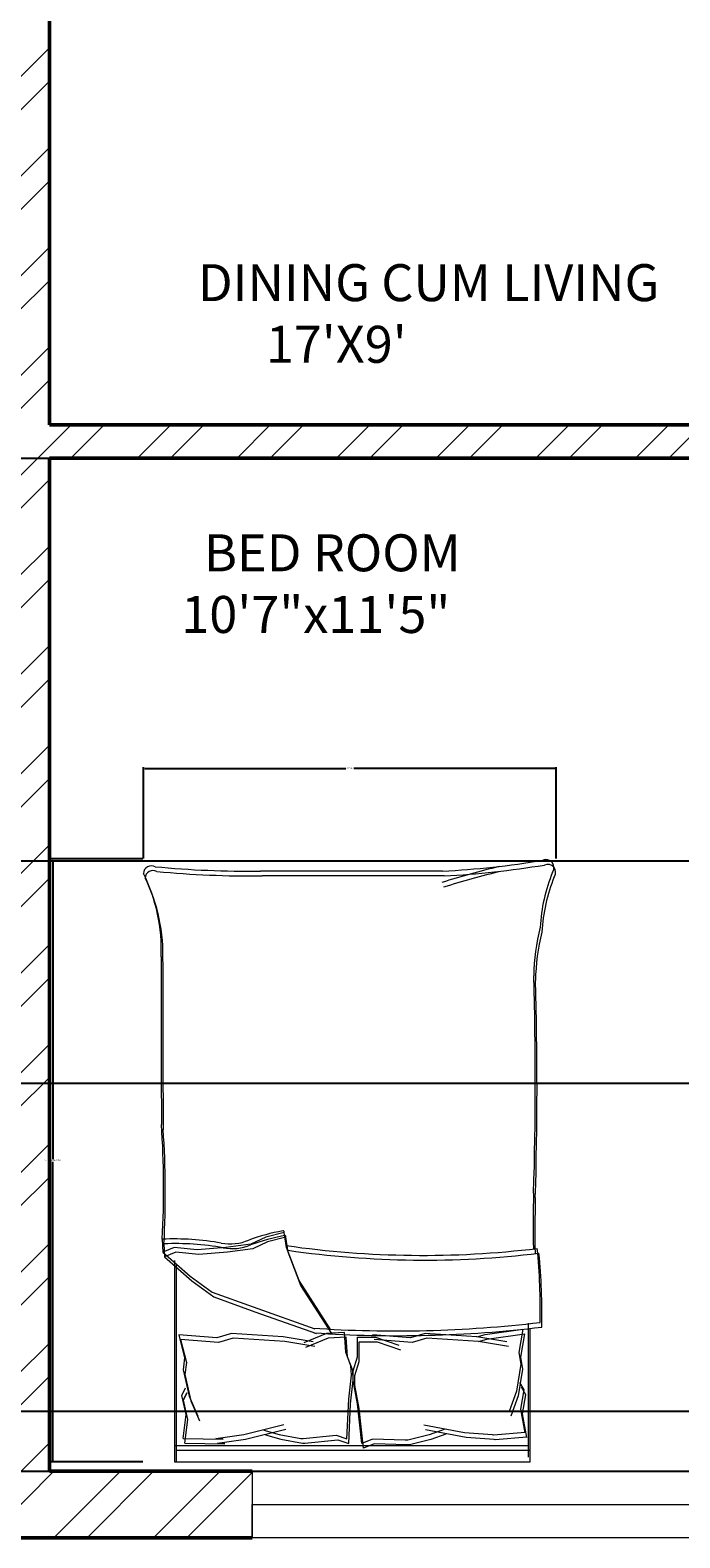
# Model space of a CAD drawing. Units: inches. Extents: x 2310 to 2937, y 1113 to 2410.
# Tile 10 of 23: x 2609 to 2697, y 1737 to 1940. Entities that reach past the tile are written whole.
import ezdxf

# ---------------------------------------------------------------- set-up
doc = ezdxf.new("R2010")
doc.units = ezdxf.units.IN
for name, color, linetype, lineweight in [('A-ANNO-DIMS', 2, 'Continuous', 18), ('A-AREA-IDEN', 7, 'Continuous', 18), ('A-FURN', 8, 'Continuous', 18), ('A-GLAZ', 191, 'Continuous', 20), ('A-WALL', 7, 'Continuous', 50), ('A-WALL-PATT', 85, 'Continuous', 13)]:
    doc.layers.add(name, color=color, linetype=linetype, lineweight=lineweight)
doc.styles.get("Standard").update_dxf_attribs({"font": 'arial.ttf'})
doc.dimstyles.get("Standard").update_dxf_attribs({"dimtxt": 0.18, "dimasz": 0.18, "dimexe": 0.18, "dimexo": 0.0625, "dimgap": 0.09, "dimtad": 0, "dimtih": 1, "dimtoh": 1, "dimdec": 4, "dimzin": 0, "dimdsep": 46, "dimtxsty": 'Standard', "dimcen": 0.09, "dimadec": 0, "dimazin": 0, "dimtfac": 1, "dimtdec": 4, "dimtofl": 0, "dimtmove": 0, "dimatfit": 3, "dimfxl": 1, "dimtolj": 1, "dimtzin": 0, "dimarcsym": 0})

# ---------------------------------------------------------------- blocks, each defined once
blk = doc.blocks.new('BED-DOUBLE')
for p, q in [((3.56, 63.44), (3.56, 81.55)), ((3.56, 63.44), (3.56, 81.55)), ((3.56, 81.55), (51.58, 81.55)), ((51.35, 81.55), (51.35, 54.94)), ((51.35, 81.55), (51.35, 54.94)), ((51.58, 81.55), (51.58, 80.91)), ((3.56, 80.01), (51.35, 80.01)), ((3.56, 80.01), (51.35, 80.01)), ((3.79, 62.8), (3.79, 80.91)), ((3.79, 62.8), (3.79, 80.91)), ((24.62, 79.1), (26.07, 79.68)), ((24.62, 79.1), (26.07, 79.68)), ((26.07, 79.68), (26.65, 74.33)), ((26.07, 79.68), (26.65, 74.33)), ((51.58, 80.91), (51.58, 54.3)), ((51.58, 80.91), (51.58, 54.3)), ((3.79, 79.38), (51.58, 79.38)), ((3.79, 79.38), (51.58, 79.38)), ((3.98, 78.21), (8.27, 78.54)), ((3.98, 78.23), (4.56, 75.05)), ((3.98, 78.23), (4.56, 75.05)), ((3.99, 78.21), (8.27, 78.54)), ((4.21, 77.57), (8.49, 77.9)), ((4.21, 77.57), (8.49, 77.9)), ((4.21, 77.59), (4.79, 74.41)), ((4.21, 77.59), (4.79, 74.41)), ((8.27, 78.54), (8.37, 78.52)), ((8.27, 78.54), (8.37, 78.52)), ((8.37, 78.52), (12.19, 78.23)), ((8.37, 78.52), (12.19, 78.23)), ((8.49, 77.9), (8.6, 77.88)), ((8.49, 77.9), (8.6, 77.88)), ((8.6, 77.88), (12.42, 77.59)), ((8.6, 77.88), (12.42, 77.59)), ((12.19, 78.23), (17.69, 77.22)), ((12.19, 78.23), (17.69, 77.22)), ((12.42, 77.59), (17.92, 76.58)), ((12.42, 77.59), (17.92, 76.58)), ((14.94, 77.8), (16.97, 78.52)), ((14.94, 77.8), (16.96, 78.52)), ((15.17, 77.16), (17.19, 77.88)), ((15.17, 77.16), (17.19, 77.88)), ((16.96, 78.52), (19.86, 79.24)), ((16.97, 78.52), (19.86, 79.24)), ((17.19, 77.88), (20.08, 78.61)), ((17.19, 77.88), (20.08, 78.61)), ((19.86, 79.24), (20.18, 79.24)), ((19.86, 79.24), (20.18, 79.24)), ((20.08, 78.61), (20.41, 78.61)), ((20.08, 78.61), (20.41, 78.61)), ((20.18, 79.24), (24.62, 79.1)), ((20.18, 79.24), (24.62, 79.1)), ((20.41, 78.61), (24.85, 78.46)), ((20.41, 78.61), (24.85, 78.46)), ((24.85, 78.46), (26.3, 79.04)), ((24.85, 78.46), (26.3, 79.04)), ((26.3, 79.04), (26.88, 73.69)), ((26.3, 79.04), (26.88, 73.69)), ((28.06, 79.06), (27.82, 73.68)), ((28.06, 79.06), (27.82, 73.68)), ((28.29, 78.42), (28.05, 73.04)), ((28.29, 78.42), (28.05, 73.04)), ((29.54, 78.57), (28.06, 79.06)), ((29.54, 78.57), (28.06, 79.06)), ((29.77, 77.93), (28.29, 78.42)), ((29.77, 77.93), (28.29, 78.42)), ((33.97, 78.99), (29.54, 78.57)), ((33.97, 78.99), (29.54, 78.57)), ((34.2, 78.35), (29.77, 77.93)), ((34.2, 78.35), (29.77, 77.93)), ((34.29, 79.01), (33.97, 78.99)), ((34.29, 79.01), (33.97, 78.99)), ((34.52, 78.37), (34.2, 78.35)), ((34.52, 78.37), (34.2, 78.35)), ((37.22, 78.47), (34.29, 79.01)), ((37.22, 78.47), (34.29, 79.01)), ((37.45, 77.83), (34.52, 78.37)), ((37.45, 77.83), (34.52, 78.37)), ((42, 78.48), (36.58, 77.13)), ((42, 78.48), (36.58, 77.13)), ((42.23, 77.84), (36.81, 76.49)), ((42.23, 77.84), (36.81, 76.49)), ((39.29, 77.87), (37.22, 78.47)), ((39.29, 77.87), (37.22, 78.47)), ((39.52, 77.24), (37.45, 77.83)), ((39.51, 77.24), (37.45, 77.83)), ((45.8, 79.01), (42, 78.48)), ((45.8, 79.01), (42, 78.48)), ((46.03, 78.37), (42.23, 77.84)), ((46.03, 78.37), (42.23, 77.84)), ((50.2, 78.99), (44.8, 79.09)), ((44.8, 79.09), (45.8, 79.01)), ((50.2, 78.99), (44.8, 79.09)), ((44.8, 79.09), (45.8, 79.01)), ((50.43, 78.35), (45.02, 78.45)), ((45.02, 78.45), (46.03, 78.37)), ((50.43, 78.35), (45.02, 78.45)), ((45.02, 78.45), (46.03, 78.37)), ((50.2, 78.99), (49.82, 75.78)), ((50.2, 78.99), (49.82, 75.78)), ((50.43, 78.35), (50.05, 75.14)), ((50.43, 78.35), (50.05, 75.14)), ((49.4, 73.29), (48.21, 75.97)), ((49.4, 73.29), (48.21, 75.97)), ((49.82, 75.78), (50.42, 73.21)), ((49.82, 75.78), (50.41, 73.21)), ((4.56, 75.05), (4.13, 72.45)), ((4.56, 75.05), (4.13, 72.45)), ((4.79, 74.41), (4.35, 71.81)), ((4.79, 74.41), (4.35, 71.81)), ((5.14, 72.59), (6.15, 75.34)), ((5.14, 72.59), (6.15, 75.34)), ((5.37, 71.95), (6.38, 74.7)), ((5.37, 71.95), (6.38, 74.7)), ((26.65, 74.33), (27.23, 71.15)), ((26.65, 74.33), (27.23, 71.15)), ((26.88, 73.69), (27.45, 70.51)), ((26.88, 73.69), (27.45, 70.51)), ((27.82, 73.68), (27.44, 70.47)), ((27.82, 73.68), (27.44, 70.47)), ((49.62, 72.65), (48.44, 75.33)), ((49.62, 72.65), (48.44, 75.33)), ((50.05, 75.14), (50.64, 72.57)), ((50.05, 75.14), (50.64, 72.57)), ((4.13, 72.45), (4.7, 71.44)), ((4.13, 72.45), (4.7, 71.44)), ((4.35, 71.81), (4.93, 70.8)), ((4.35, 71.81), (4.93, 70.8)), ((4.56, 68.98), (5.14, 72.59)), ((4.56, 68.98), (5.14, 72.59)), ((4.79, 68.34), (5.37, 71.95)), ((4.79, 68.34), (5.37, 71.95)), ((28.05, 73.04), (27.67, 69.83)), ((28.05, 73.04), (27.67, 69.83)), ((50.2, 69.72), (49.4, 73.29)), ((50.2, 69.72), (49.4, 73.29)), ((50.43, 69.08), (49.62, 72.65)), ((50.43, 69.08), (49.62, 72.65)), ((50.42, 73.21), (49.9, 72.16)), ((50.41, 73.21), (49.9, 72.16)), ((50.64, 72.57), (50.13, 71.52)), ((50.64, 72.57), (50.13, 71.52)), ((27.23, 69.85), (26.65, 67.97)), ((27.23, 69.85), (26.65, 67.97)), ((27.23, 71.15), (27.23, 69.85)), ((27.23, 71.15), (27.23, 69.85)), ((27.44, 70.47), (27.52, 69.17)), ((27.44, 70.47), (27.52, 69.17)), ((27.45, 70.51), (27.45, 69.21)), ((27.45, 70.51), (27.45, 69.21)), ((27.67, 69.83), (27.75, 68.53)), ((27.67, 69.83), (27.75, 68.53)), ((50.01, 68.11), (50.2, 69.72)), ((50.01, 68.11), (50.2, 69.72)), ((4.27, 64.21), (4.85, 67.39)), ((4.27, 64.21), (4.85, 67.39)), ((4.85, 67.39), (4.56, 68.98)), ((4.85, 67.39), (4.56, 68.98)), ((5.08, 66.75), (4.79, 68.34)), ((5.08, 66.75), (4.79, 68.34)), ((26.65, 67.97), (26.65, 65.29)), ((26.65, 67.97), (26.65, 65.29)), ((27.45, 69.21), (26.88, 67.33)), ((27.45, 69.21), (26.88, 67.33)), ((26.88, 67.33), (26.88, 64.65)), ((26.88, 67.33), (26.88, 64.65)), ((27.52, 69.17), (28.22, 67.33)), ((27.52, 69.17), (28.22, 67.33)), ((27.75, 68.53), (28.45, 66.69)), ((27.75, 68.53), (28.44, 66.69)), ((28.22, 67.33), (28.38, 64.66)), ((28.22, 67.33), (28.38, 64.66)), ((50.78, 64.98), (50.01, 68.11)), ((50.78, 64.98), (50.01, 68.11)), ((50.24, 67.48), (50.43, 69.08)), ((50.24, 67.48), (50.43, 69.08)), ((51.01, 64.34), (50.24, 67.48)), ((51.01, 64.34), (50.24, 67.48)), ((4.5, 63.57), (5.08, 66.75)), ((4.5, 63.57), (5.08, 66.75)), ((6.47, 65.92), (10.5, 65.25)), ((6.47, 65.92), (10.5, 65.25)), ((6.7, 65.28), (10.73, 64.61)), ((6.7, 65.28), (10.73, 64.61)), ((10.5, 65.25), (9.37, 64.93)), ((10.5, 65.25), (9.37, 64.93)), ((10.5, 65.25), (17.51, 64.82)), ((10.5, 65.25), (17.51, 64.82)), ((17.51, 64.82), (19.47, 65.38)), ((17.51, 64.82), (19.47, 65.38)), ((19.47, 65.38), (24.6, 64.98)), ((19.47, 65.38), (24.6, 64.98)), ((24.19, 65.29), (21.04, 66.38)), ((24.19, 65.29), (21.05, 66.38)), ((24.42, 64.65), (21.27, 65.74)), ((24.42, 64.65), (21.27, 65.74)), ((26.65, 65.29), (24.19, 65.29)), ((26.65, 65.29), (24.19, 65.29)), ((28.44, 66.69), (28.61, 64.02)), ((28.45, 66.69), (28.61, 64.02)), ((30.84, 64.81), (33.91, 66.09)), ((30.84, 64.81), (33.91, 66.09)), ((31.06, 64.17), (34.14, 65.45)), ((31.07, 64.17), (34.14, 65.45)), ((32.65, 65.92), (36.68, 65.25)), ((32.65, 65.92), (36.68, 65.25)), ((32.88, 65.28), (36.91, 64.61)), ((32.88, 65.28), (36.91, 64.61)), ((36.68, 65.25), (43.69, 64.82)), ((36.68, 65.25), (43.69, 64.82)), ((43.69, 64.82), (45.65, 65.38)), ((43.69, 64.82), (45.65, 65.38)), ((45.65, 65.38), (50.78, 64.98)), ((45.65, 65.38), (50.78, 64.98)), ((9.37, 64.93), (4.27, 64.21)), ((9.37, 64.93), (4.27, 64.21)), ((9.6, 64.29), (4.5, 63.57)), ((9.6, 64.29), (4.5, 63.57)), ((10.73, 64.61), (9.6, 64.29)), ((10.73, 64.61), (9.6, 64.29)), ((10.73, 64.61), (17.74, 64.18)), ((10.73, 64.61), (17.74, 64.18)), ((17.74, 64.18), (19.7, 64.74)), ((17.74, 64.18), (19.7, 64.74)), ((19.7, 64.74), (24.83, 64.34)), ((19.7, 64.74), (24.83, 64.34)), ((26.88, 64.65), (24.42, 64.65)), ((26.88, 64.65), (24.42, 64.65)), ((28.38, 64.66), (30.84, 64.81)), ((28.38, 64.66), (30.84, 64.81)), ((28.61, 64.02), (31.07, 64.17)), ((28.61, 64.02), (31.06, 64.17)), ((30.35, 64.17), (34.54, 57.67)), ((30.35, 64.17), (34.54, 57.67)), ((30.57, 63.53), (34.76, 57.03)), ((30.57, 63.53), (34.76, 57.03)), ((40.73, 61.23), (32.39, 64.17)), ((40.73, 61.23), (32.39, 64.17)), ((40.96, 60.59), (32.62, 63.53)), ((40.96, 60.59), (32.62, 63.53)), ((36.91, 64.61), (43.92, 64.18)), ((36.91, 64.61), (43.92, 64.18)), ((43.92, 64.18), (45.88, 64.74)), ((43.92, 64.18), (45.88, 64.74)), ((45.88, 64.74), (51.01, 64.34)), ((45.88, 64.74), (51.01, 64.34)), ((46.31, 59.22), (40.73, 61.23)), ((46.31, 59.22), (40.73, 61.23)), ((46.53, 58.58), (40.96, 60.59)), ((46.53, 58.58), (40.96, 60.59)), ((49.25, 57.05), (46.31, 59.22)), ((49.25, 57.05), (46.31, 59.22)), ((34.54, 57.67), (36.24, 53.18)), ((34.54, 57.67), (36.24, 53.18)), ((49.48, 56.41), (46.53, 58.58)), ((49.48, 56.41), (46.53, 58.58)), ((34.76, 57.03), (36.47, 52.54)), ((34.76, 57.03), (36.47, 52.54)), ((52.95, 53.8), (49.25, 57.05)), ((52.95, 53.8), (49.25, 57.05)), ((53.18, 53.16), (49.48, 56.41)), ((53.18, 53.16), (49.48, 56.41)), ((36.24, 53.18), (36.55, 51.17)), ((36.24, 53.18), (36.55, 51.17)), ((41.04, 52.72), (44.45, 53.18)), ((41.04, 52.72), (44.45, 53.18)), ((44.45, 53.18), (48.32, 53.49)), ((44.45, 53.18), (48.32, 53.49)), ((48.32, 53.49), (51.42, 53.18)), ((48.32, 53.49), (51.42, 53.18)), ((51.42, 53.18), (52.95, 53.8)), ((51.42, 53.18), (52.95, 53.8)), ((51.65, 52.54), (53.18, 53.16)), ((51.65, 52.54), (53.18, 53.16)), ((53.03, 52.06), (52.95, 53.8, 3.87)), ((53.03, 52.06), (52.95, 53.8, 3.87)), ((53.26, 51.42), (53.18, 53.16, 3.87)), ((53.26, 51.42), (53.18, 53.16, 3.87)), ((36.47, 52.54), (36.78, 50.53)), ((36.47, 52.54), (36.78, 50.53)), ((36.55, 51.17), (39.03, 51.79)), ((36.55, 51.17), (39.03, 51.79)), ((36.78, 50.53), (39.26, 51.15)), ((36.78, 50.53), (39.26, 51.15)), ((39.03, 51.79), (41.04, 52.72)), ((39.03, 51.79), (41.04, 52.72)), ((39.26, 51.15), (41.27, 52.08)), ((39.26, 51.15), (41.27, 52.08)), ((41.27, 52.08), (44.68, 52.54)), ((41.27, 52.08), (44.68, 52.54)), ((44.68, 52.54), (48.55, 52.85)), ((44.68, 52.54), (48.55, 52.85)), ((48.55, 52.85), (51.65, 52.54)), ((48.55, 52.85), (51.65, 52.54)), ((15.15, 2.3), (39.76, 2.3)), ((15.15, 2.3), (39.76, 2.3)), ((15.38, 1.66), (39.99, 1.66)), ((15.38, 1.66), (39.99, 1.66))]:
    blk.add_line(p, q)
for centre, radius, start, end in [((85.25, 61.45), 83.31, 178.7218, 185.604), ((85.25, 61.45), 83.31, 178.7218, 185.604), ((21.45, -100.5), 164.97, 86.0865, 96.7821), ((21.45, -100.5), 164.97, 86.0865, 96.7821), ((21.67, -101.14), 164.97, 86.0865, 96.7821), ((21.67, -101.14), 164.97, 86.0865, 96.7821), ((85.48, 60.81), 83.31, 178.7218, 185.604), ((85.48, 60.81), 83.31, 178.7218, 185.604), ((17.84, -74.77), 129.02, 81.7845, 96.9006), ((17.84, -74.77), 129.02, 81.7845, 96.9006), ((18.07, -75.41), 129.02, 81.7845, 96.9006), ((18.07, -75.41), 129.02, 81.7845, 96.9006), ((-167.22, 50.37), 170.11, 358.4762, 1.0082), ((-167.22, 50.37), 170.11, 358.4762, 1.0082), ((-166.99, 49.74), 170.11, 358.4762, 1.0082), ((-166.99, 49.74), 170.11, 358.4762, 1.0082), ((36.72, 51.11), 0.185, 160.2464, 271.1377), ((36.72, 51.11), 0.185, 160.2464, 271.1377), ((31.24, 80.07), 29.65, 280.6617, 289.8806), ((31.24, 80.07), 29.65, 280.6617, 289.8806), ((31.47, 79.43), 29.65, 280.6617, 289.8806), ((31.47, 79.43), 29.65, 280.6617, 289.8806), ((43.83, 46.48), 6.22, 78.6608, 113.7384), ((43.83, 46.48), 6.22, 78.6608, 113.7384), ((44.06, 45.84), 6.22, 78.6608, 113.7384), ((44.06, 45.84), 6.22, 78.6608, 113.7384), ((51.41, 88.2), 36.18, 259.8763, 272.5657), ((51.41, 88.2), 36.18, 259.8763, 272.5657), ((51.64, 87.57), 36.18, 259.8763, 272.5657), ((51.64, 87.57), 36.18, 259.8763, 272.5657), ((182.35, 45.23), 129.5, 176.9791, 183.8365), ((182.35, 45.23), 129.5, 176.9791, 183.8365), ((182.58, 44.59), 129.5, 176.9791, 183.8365), ((182.58, 44.59), 129.5, 176.9791, 183.8365), ((36.95, 50.47), 0.185, 160.2464, 271.1377), ((36.95, 50.47), 0.185, 160.2464, 271.1377), ((484.91, 30.93), 482.31, 178.2277, 181.7185), ((484.91, 30.93), 482.31, 178.2277, 181.7185), ((485.14, 30.3), 482.31, 178.2277, 181.7185), ((485.14, 30.3), 482.31, 178.2277, 181.7185), ((-4508.66, 13.73), 4561.86, 0.00217, 0.28689), ((-4508.66, 13.73), 4561.86, 0.00217, 0.28689), ((-4508.43, 13.09), 4561.86, 0.00217, 0.28689), ((-4508.43, 13.09), 4561.86, 0.00217, 0.28689), ((-26.81, 17.03), 29.63, 346.0648, 358.9113), ((-26.81, 17.03), 29.63, 346.0648, 358.9113), ((-26.58, 16.39), 29.63, 346.0648, 358.9113), ((-26.58, 16.39), 29.63, 346.0648, 358.9113), ((76.24, 12.88), 23.07, 177.4714, 206.4681), ((76.24, 12.88), 23.07, 177.4714, 206.4681), ((76.47, 12.24), 23.07, 177.4714, 206.4681), ((76.47, 12.24), 23.07, 177.4714, 206.4681), ((-21.57, 11.27), 23.56, 337.9751, 356.652), ((-21.57, 11.27), 23.56, 337.9751, 356.652), ((-21.34, 10.63), 23.56, 337.9751, 356.652), ((-21.34, 10.63), 23.56, 337.9751, 356.652), ((1.17, 1.83), 1.09, 146.1736, 293.4781), ((1.17, 1.83), 1.09, 146.1736, 293.4781), ((21.51, -119.29), 121.76, 92.9958, 99.4091), ((21.51, -119.29), 121.76, 92.9958, 99.4091), ((-17.14, 105.26), 106.46, 283.3832, 287.7053), ((-17.14, 105.26), 106.46, 283.3832, 287.7053), ((-16.91, 104.62), 106.46, 283.3832, 287.7053), ((-16.91, 104.62), 106.46, 283.3832, 287.7053), ((41.24, -130.73), 133.04, 84.4998, 90.6351), ((41.24, -130.73), 133.04, 84.4998, 90.6351), ((54.5, 2.68), 1.1, 242.6588, 356.02), ((54.5, 2.68), 1.1, 242.6588, 356.02), ((1.4, 1.19), 1.09, 146.1736, 293.4781), ((1.4, 1.19), 1.09, 146.1736, 293.4781), ((21.74, -119.93), 121.76, 92.9958, 99.4091), ((21.74, -119.93), 121.76, 92.9958, 99.4091), ((41.47, -131.37), 133.04, 84.4998, 90.6351), ((41.47, -131.37), 133.04, 84.4998, 90.6351), ((54.72, 2.04), 1.1, 242.6588, 356.02), ((54.72, 2.04), 1.1, 242.6588, 356.02)]:
    blk.add_arc(centre, radius, start, end)
blk = doc.blocks.new('WIN-60IN')
for p, q in [((4.5, 60), (0, 60)), ((0, 60), (9, 60)), ((0, 60), (0, 0)), ((4.5, 0), (4.5, 60)), ((9, 60), (9, 0)), ((0, 0), (9, 0)), ((9, 0), (4.5, 0))]:
    blk.add_line(p, q)
blk = doc.blocks.new('*D35')
at = {"layer": 'A-ANNO-DIMS', "color": 0, "lineweight": -2, "transparency": 16777216}
for p, q in [((2624.13, 1828.32), (2611.78, 1828.32)), ((2611.96, 1828.14), (2611.96, 1787.73)), ((2611.96, 1746.95), (2611.96, 1787.36)), ((2624.13, 1746.77), (2611.78, 1746.77))]:
    blk.add_line(p, q, dxfattribs=at)
at = {"layer": 'A-ANNO-DIMS', "color": 0, "transparency": 16777216}
for points in [[(2611.93, 1828.14), (2611.99, 1828.14), (2611.96, 1828.32)], [(2611.93, 1746.95), (2611.99, 1746.95), (2611.96, 1746.77)]]:
    blk.add_solid(points, dxfattribs=at)
at = {"layer": 'Defpoints', "color": 0, "transparency": 16777216}
for p in [(2624.19, 1828.32), (2611.96, 1746.77), (2624.19, 1746.77)]:
    blk.add_point(p, dxfattribs=at)
at = {"layer": 'A-ANNO-DIMS', "color": 0, "transparency": 16777216, "insert": (2611.96, 1787.54), "char_height": 0.18, "attachment_point": 5}
blk.add_mtext('\\A1;DOUBLE BED 82 TYP.', dxfattribs=at)
blk = doc.blocks.new('*D36')
at = {"layer": 'A-ANNO-DIMS', "color": 0, "lineweight": -2, "transparency": 16777216}
for p, q in [((2624.19, 1828.38), (2624.19, 1840.73)), ((2624.37, 1840.55), (2651.57, 1840.55)), ((2679.83, 1840.55), (2652.63, 1840.55)), ((2680.01, 1828.38), (2680.01, 1840.73))]:
    blk.add_line(p, q, dxfattribs=at)
at = {"layer": 'A-ANNO-DIMS', "color": 0, "transparency": 16777216}
for points in [[(2624.37, 1840.58), (2624.37, 1840.52), (2624.19, 1840.55)], [(2679.83, 1840.58), (2679.83, 1840.52), (2680.01, 1840.55)]]:
    blk.add_solid(points, dxfattribs=at)
at = {"layer": 'Defpoints', "color": 0, "transparency": 16777216}
for p in [(2624.19, 1840.55), (2624.19, 1828.32), (2680.01, 1828.32)]:
    blk.add_point(p, dxfattribs=at)
at = {"layer": 'A-ANNO-DIMS', "color": 0, "transparency": 16777216, "insert": (2652.1, 1840.55), "char_height": 0.18, "attachment_point": 5}
blk.add_mtext('\\A1;56 TYP.', dxfattribs=at)
blk = doc.blocks.new('*D55')
at = {"layer": 'A-ANNO-DIMS', "color": 0, "lineweight": -2, "transparency": 16777216}
for p, q in [((2403.55, 1753.64), (2858.02, 1753.64)), ((2857.84, 1753.46), (2857.84, 1749.76)), ((2857.84, 1745.69), (2857.84, 1749.4)), ((2403.55, 1745.51), (2858.02, 1745.51))]:
    blk.add_line(p, q, dxfattribs=at)
at = {"layer": 'A-ANNO-DIMS', "color": 0, "transparency": 16777216}
for points in [[(2857.81, 1753.46), (2857.87, 1753.46), (2857.84, 1753.64)], [(2857.81, 1745.69), (2857.87, 1745.69), (2857.84, 1745.51)]]:
    blk.add_solid(points, dxfattribs=at)
at = {"layer": 'Defpoints', "color": 0, "transparency": 16777216}
for p in [(2403.49, 1753.64), (2857.84, 1753.64), (2403.49, 1745.51)]:
    blk.add_point(p, dxfattribs=at)
at = {"layer": 'A-ANNO-DIMS', "color": 0, "transparency": 16777216, "insert": (2857.84, 1749.58), "char_height": 0.18, "attachment_point": 5}
blk.add_mtext('\\A1;8.127', dxfattribs=at)
blk = doc.blocks.new('*D56')
at = {"layer": 'A-ANNO-DIMS', "color": 0, "lineweight": -2, "transparency": 16777216}
for p, q in [((2403.55, 1828.04), (2858.02, 1828.04)), ((2857.84, 1827.86), (2857.84, 1813.21)), ((2857.84, 1798.19), (2857.84, 1812.85)), ((2403.55, 1798.01), (2858.02, 1798.01))]:
    blk.add_line(p, q, dxfattribs=at)
at = {"layer": 'A-ANNO-DIMS', "color": 0, "transparency": 16777216}
for points in [[(2857.81, 1827.86), (2857.87, 1827.86), (2857.84, 1828.04)], [(2857.81, 1798.19), (2857.87, 1798.19), (2857.84, 1798.01)]]:
    blk.add_solid(points, dxfattribs=at)
at = {"layer": 'Defpoints', "color": 0, "transparency": 16777216}
for p in [(2403.49, 1828.04), (2857.84, 1828.04), (2403.49, 1798.01)]:
    blk.add_point(p, dxfattribs=at)
at = {"layer": 'A-ANNO-DIMS', "color": 0, "transparency": 16777216, "insert": (2857.84, 1813.03), "char_height": 0.18, "attachment_point": 5}
blk.add_mtext('\\A1;30.03', dxfattribs=at)
blk = doc.blocks.new('*D58')
at = {"layer": 'A-ANNO-DIMS', "color": 0, "lineweight": -2, "transparency": 16777216}
for p, q in [((2475.55, 1882.51), (2858.02, 1882.51)), ((2857.84, 1882.33), (2857.84, 1840.45)), ((2857.84, 1798.19), (2857.84, 1840.08)), ((2475.55, 1798.01), (2858.02, 1798.01))]:
    blk.add_line(p, q, dxfattribs=at)
at = {"layer": 'A-ANNO-DIMS', "color": 0, "transparency": 16777216}
for points in [[(2857.81, 1882.33), (2857.87, 1882.33), (2857.84, 1882.51)], [(2857.81, 1798.19), (2857.87, 1798.19), (2857.84, 1798.01)]]:
    blk.add_solid(points, dxfattribs=at)
at = {"layer": 'Defpoints', "color": 0, "transparency": 16777216}
for p in [(2475.49, 1882.51), (2857.84, 1882.51), (2475.49, 1798.01)]:
    blk.add_point(p, dxfattribs=at)
at = {"layer": 'A-ANNO-DIMS', "color": 0, "transparency": 16777216, "insert": (2857.84, 1840.26), "char_height": 0.18, "attachment_point": 5}
blk.add_mtext('\\A1;84.5', dxfattribs=at)

msp = doc.modelspace()

# ---------------------------------------------------------------- hatches: boundary and pattern name
at = {"layer": 'A-WALL-PATT'}
h = msp.add_hatch(dxfattribs=at)
h.set_pattern_fill('ANSI32', color=256)
h.paths.add_polyline_path([(2639.1394, 2356.5139), (2563.662, 2356.5139), (2563.662, 2347.5139), (2606.9859, 2347.5139), (2606.9859, 2210.5139), (2514.2692, 2210.5139), (2514.2692, 2206.0139), (2606.9859, 2206.0139), (2606.9859, 2098.0139), (2602.689, 2098.0139), (2602.689, 2093.5139), (2615.5262, 2093.5139), (2615.5262, 2095.7639), (2615.5262, 2098.0139), (2611.4859, 2098.0139), (2611.4859, 2206.0139), (2703.9391, 2206.0139), (2703.9391, 2208.2639), (2703.9391, 2210.5139), (2611.4859, 2210.5139), (2611.4859, 2347.5139), (2639.1394, 2347.5139)])
h.paths.add_polyline_path([(2823.9859, 2356.5139), (2699.1394, 2356.5139), (2699.1394, 2347.5139), (2738.4859, 2347.5139), (2738.4859, 2343.9266), (2742.9859, 2343.9266), (2742.9859, 2347.5139), (2814.9859, 2347.5139), (2814.9859, 2336.76), (2823.9859, 2336.76)])
h.paths.add_polyline_path([(2823.9859, 2312.76), (2814.9859, 2312.76), (2814.9859, 2299.5139), (2742.9859, 2299.5139), (2742.9859, 2323.0159), (2740.7359, 2323.0159), (2738.4859, 2323.0159), (2738.4859, 2210.5139), (2734.5483, 2210.5139), (2734.5483, 2206.0139), (2746.8769, 2206.0139), (2746.8769, 2208.2639), (2746.8769, 2210.5139), (2742.9859, 2210.5139), (2742.9859, 2295.0139), (2814.9859, 2295.0139), (2814.9859, 2269.8977), (2823.9859, 2269.8977)])
h.paths.add_polyline_path([(2823.9859, 2210.5139), (2823.9859, 2233.8977), (2819.4859, 2233.8977), (2814.9859, 2233.8977), (2814.9859, 2210.5139), (2769.9745, 2210.5139), (2769.9745, 2206.0139), (2814.9859, 2206.0139), (2814.9859, 2178.3027), (2823.9859, 2178.3027)])
h.paths.add_polyline_path([(2823.9859, 2118.3027), (2819.4859, 2118.3027), (2814.9859, 2118.3027), (2814.9859, 2098.0139), (2647.0333, 2098.0139), (2647.0333, 2093.5139), (2814.9859, 2093.5139), (2814.9859, 1999.5139), (2650.6052, 1999.5139), (2650.6052, 1995.0139), (2814.9859, 1995.0139), (2814.9859, 1969.9784), (2823.9859, 1969.9784)])
h.paths.add_polyline_path([(2403.4859, 2093.5139), (2569.9888, 2093.5139), (2569.9888, 2095.7639), (2569.9888, 2098.0139), (2403.4859, 2098.0139), (2403.4859, 2131.7587), (2394.4859, 2131.7587), (2394.4859, 1967.522), (2403.4859, 1967.522), (2403.4859, 1995.0139), (2569.8903, 1995.0139), (2569.8903, 1997.2639), (2569.8903, 1999.5139), (2403.4859, 1999.5139)])
h.paths.add_polyline_path([(2503.662, 2356.5139), (2394.4859, 2356.5139), (2394.4859, 2337.9231), (2398.9859, 2337.9231), (2403.4859, 2337.9231), (2403.4859, 2347.5139), (2475.4859, 2347.5139), (2475.4859, 2343.0384), (2479.9859, 2343.0384), (2479.9859, 2347.5139), (2503.662, 2347.5139)])
h.paths.add_polyline_path([(2498.3065, 1745.5139), (2479.9859, 1745.5139), (2479.9859, 1749.1663), (2477.7359, 1749.1663), (2475.4859, 1749.1663), (2475.4859, 1745.5139), (2403.4859, 1745.5139), (2403.4859, 1753.6409), (2398.9859, 1753.6409), (2394.4859, 1753.6409), (2394.4859, 1736.5139), (2498.3065, 1736.5139), (2498.3065, 1741.0139)])
h.paths.add_polyline_path([(2479.9859, 1882.5139), (2483.9367, 1882.5139), (2483.9367, 1887.0139), (2471.5501, 1887.0139), (2471.5501, 1885.1969), (2471.5501, 1882.5139), (2475.4859, 1882.5139), (2475.4859, 1798.0139), (2403.4859, 1798.0139), (2403.4859, 1828.0433), (2402.2852, 1828.0433), (2394.4859, 1828.0433), (2394.4859, 1777.6409), (2403.4859, 1777.6409), (2403.4859, 1793.5139), (2475.4859, 1793.5139), (2475.4859, 1769.1696), (2479.9859, 1769.1696)])
h.paths.add_polyline_path([(2403.4859, 1907.522), (2398.9859, 1907.522), (2394.4859, 1907.522), (2394.4859, 1864.0433), (2403.4859, 1864.0433), (2403.4859, 1882.5139), (2448.9325, 1882.5139), (2448.9325, 1884.7639), (2448.9325, 1887.0139), (2403.4859, 1887.0139)])
h.paths.add_polyline_path([(2702.2061, 1887.0139), (2611.4859, 1887.0139), (2611.4859, 1995.0139), (2615.6132, 1995.0139), (2615.6132, 1999.5139), (2602.4798, 1999.5139), (2602.4798, 1997.2639), (2602.4798, 1995.0139), (2606.9859, 1995.0139), (2606.9859, 1887.0139), (2516.2443, 1887.0139), (2516.2443, 1884.7639), (2516.2443, 1882.5139), (2606.9859, 1882.5139), (2606.9859, 1745.5139), (2558.3065, 1745.5139), (2558.3065, 1736.5139), (2638.8921, 1736.5139), (2638.8921, 1741.0139), (2638.8921, 1745.5139), (2611.4859, 1745.5139), (2611.4859, 1882.5139), (2702.2061, 1882.5139)])
h.paths.add_polyline_path([(2823.9859, 1909.9784), (2819.4859, 1909.9784), (2814.9859, 1909.9784), (2814.9859, 1887.0139), (2769.144, 1887.0139), (2769.144, 1884.7639), (2769.144, 1882.5139), (2814.9859, 1882.5139), (2814.9859, 1854.1704), (2823.9859, 1854.1704)])
h.paths.add_polyline_path([(2823.9859, 1818.1704), (2819.4859, 1818.1704), (2814.9859, 1818.1704), (2814.9859, 1798.0139), (2742.9859, 1798.0139), (2742.9859, 1882.5139), (2746.805, 1882.5139), (2746.805, 1887.0139), (2733.7334, 1887.0139), (2733.7334, 1884.7639), (2733.7334, 1882.5139), (2738.4859, 1882.5139), (2738.4859, 1771.1728), (2740.7359, 1771.1728), (2742.9859, 1771.1728), (2742.9859, 1793.5139), (2814.9859, 1793.5139), (2814.9859, 1783.6684), (2823.9859, 1783.6684)])
h.paths.add_polyline_path([(2823.9859, 1759.6684), (2814.9859, 1759.6684), (2814.9859, 1745.5139), (2742.9859, 1745.5139), (2742.9859, 1748.9831), (2740.7359, 1748.9831), (2738.4859, 1748.9831), (2738.4859, 1745.5139), (2698.8921, 1745.5139), (2698.8921, 1736.5139), (2823.9859, 1736.5139)])

# ---------------------------------------------------------------- linework, layer by layer
at = {"layer": 'A-WALL'}
for p, q in [((2611.4859, 1995.0139), (2611.4859, 1887.0139)), ((2611.4859, 1887.0139), (2702.2061, 1887.0139)), ((2611.4859, 1882.5139), (2703.6918, 1882.5139)), ((2611.4859, 1882.5139), (2611.4859, 1745.5139)), ((2611.4859, 1745.5139), (2638.8921, 1745.5139)), ((2558.3065, 1736.5139), (2638.8921, 1736.5139))]:
    msp.add_line(p, q, dxfattribs=at)

# ---------------------------------------------------------------- block references
at = {"layer": 'A-FURN', "rotation": 180}
msp.add_blockref('BED-DOUBLE', (2680.0124, 1828.3177), dxfattribs=at)
at = {"layer": 'A-GLAZ', "rotation": 270}
msp.add_blockref('WIN-60IN', (2638.8921, 1745.5139), dxfattribs=at)

# ---------------------------------------------------------------- texts
at = {"layer": 'A-AREA-IDEN', "char_height": 5, "attachment_point": 1}
for s, width, insert in [("      DINING CUM LIVING\\P            17'X9'", 162.169763, (2622.4091, 1908.7241)), ('    BED ROOM\\P  10\'7"x11\'5"', 124.75424, (2626.2628, 1872.1961))]:
    msp.add_mtext_dynamic_manual_height_columns(s, width=width, gutter_width=12.5, heights=[0], dxfattribs=dict(at, insert=insert))

# ---------------------------------------------------------------- dimensions: what is measured, and where the dimension line sits
at = {"layer": 'A-ANNO-DIMS'}
for base, p1, p2, override, picture, middle in [((2857.8359, 1882.5139), (2475.4859, 1798.0139), (2475.4859, 1882.5139), {"dimdec": 1, "dimlfac": 1, "dimrnd": 0, "dimzin": 0, "dimdsep": 46, "dimlunit": 2}, '*D58', (2857.8359, 1840.2639)), ((2857.8359, 1828.0433), (2403.4859, 1798.0139), (2403.4859, 1828.0433), {"dimdec": 2, "dimlfac": 1, "dimrnd": 0, "dimzin": 0, "dimdsep": 46, "dimlunit": 2}, '*D56', (2857.8359, 1813.0286)), ((2857.8359, 1753.6409), (2403.4859, 1745.5139), (2403.4859, 1753.6409), {"dimdec": 3, "dimlfac": 1, "dimrnd": 0, "dimzin": 0, "dimdsep": 46, "dimlunit": 2}, '*D55', (2857.8359, 1749.5774))]:
    dim = msp.add_linear_dim(base=base, p1=p1, p2=p2, angle=90, dimstyle='Standard', override=override, dxfattribs=at)
    dim.commit()
    dim.dimension.update_dxf_attribs({"geometry": picture, "text_midpoint": middle})
for base, p1, p2, angle, text, picture, middle in [((2624.1879, 1840.55), (2680.0124, 1828.3177), (2624.1879, 1828.3177), 180, '<> TYP.', '*D36', (2652.1001, 1840.55)), ((2611.9556, 1746.7691), (2624.1879, 1828.3177), (2624.1879, 1746.7691), 270, 'DOUBLE BED <> TYP.', '*D35', (2611.9556, 1787.5434))]:
    dim = msp.add_linear_dim(base=base, p1=p1, p2=p2, angle=angle, text=text, dimstyle='Standard', override={"dimdec": 0, "dimlfac": 1, "dimrnd": 0, "dimzin": 0, "dimdsep": 46, "dimlunit": 2}, dxfattribs=at)
    dim.commit()
    dim.dimension.update_dxf_attribs({"geometry": picture, "text_midpoint": middle})

doc.saveas('drawing.dxf')
